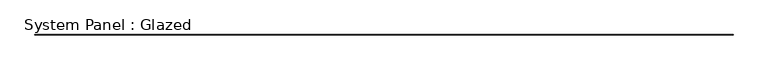
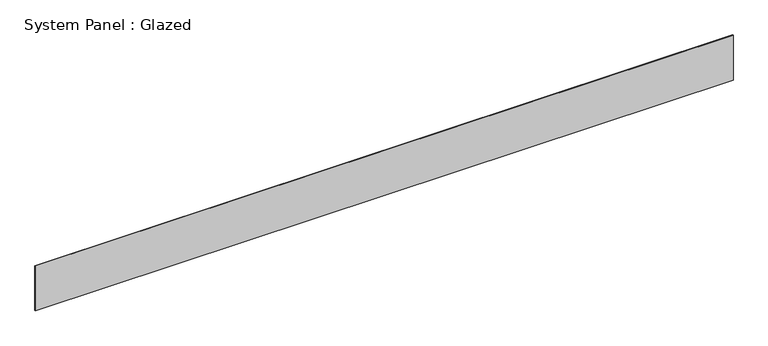
"""IFC4 building model written with IfcOpenShell, lengths in millimetres: plate geometry, System Panel : Glazed."""

from ifc_helpers import new_model, si_unit, origin, origin_with_axes, place, context, project, spatial, polyline, outline, extrude, source, transform, mapped, element, save


def system_panel_glazed_f2f268b4(model_context):
    return source(origin(), model_context, "Body", "SweptSolid", [
        extrude(outline(polyline([(15773.4, 19.05), (-15773.4, 19.05), (-15773.4, 44.45), (15773.4, 44.45), (15773.4, 19.05)])), origin_with_axes(), (0.0, 0.0, 1.0), 2141.8122839),
    ])


if __name__ == "__main__":
    model = new_model("IFC4")
    model_context = context("Model", 3, world=origin())
    ifc_project = project(units=[si_unit("LENGTHUNIT", "METRE", prefix="MILLI")], contexts=[model_context])
    site = spatial("IfcSite", under=ifc_project)
    building = spatial("IfcBuilding", under=site)
    placement = place(None, origin())
    system_panel_glazed_shape = system_panel_glazed_f2f268b4(model_context)
    element("IfcPlate", 1, ObjectType="System Panel : Glazed", at=placement, inside=building, context=model_context, shape_type="MappedRepresentation", body=[
        mapped(system_panel_glazed_shape, transform((0.0, 0.0, 0.0), x_axis=(1.0, 0.0, 0.0), y_axis=(0.0, 1.0, 0.0), z_axis=(0.0, 0.0, 1.0))),
    ])
    save(model, "model.ifc")

# Revit data of these elements
# Type "System Panel : Glazed"
#   Construction Type Id = "GSP4R"
#   Analytic Construction = "1/8 in Pilkington single glazing"
#   Visual Light Transmittance = 0.9
#   Solar Heat Gain Coefficient = 0.86
#   Heat Transfer Coefficient (U) = 1.18115 BTU/(h·ft²·°F)
# Element 1 (IfcPlate, "System Panel : Glazed")
#   Materials on its faces: "Glass"
# Materials
#   "Glass": class "Glass", colour RGB 0 128 192, transparency 0.75, Description = "Soda Lime Glass", Cost = 0
